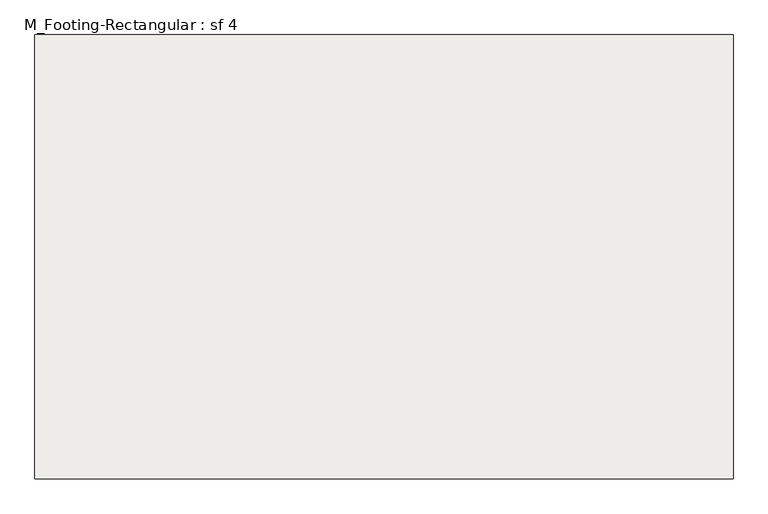
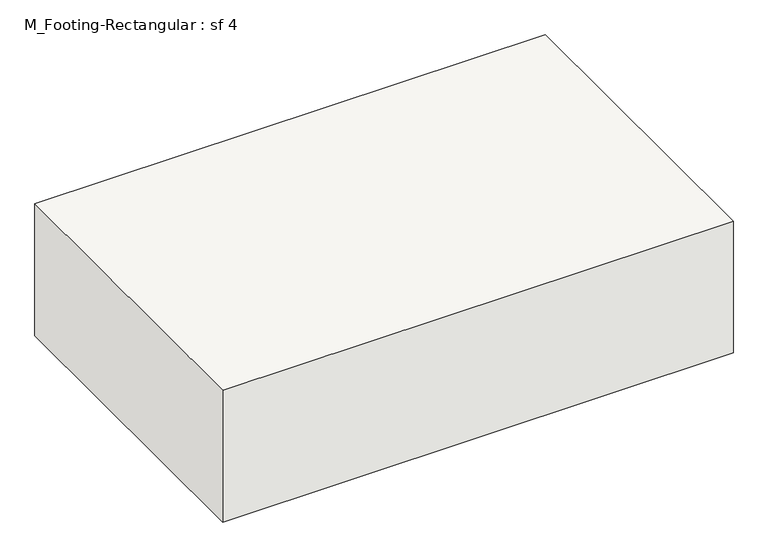
"""IFC4 building model written with IfcOpenShell, lengths in millimetres: slab geometry, M_Footing-Rectangular : sf 4."""

from ifc_helpers import new_model, si_unit, frame, origin, place, context, project, spatial, polyline, outline, extrude, source, transform, mapped, element, save


def m_footing_rectangular_sf_4_edbcb53e(model_context):
    return source(origin(), model_context, "Body", "SweptSolid", [
        extrude(outline(polyline([(838.2, 533.4), (838.2, -533.4), (-838.2, -533.4), (-838.2, 533.4), (838.2, 533.4)])), frame((0.0, 0.0, -457.2), z_axis=(0.0, 0.0, 1.0), x_axis=(1.0, 0.0, 0.0)), (0.0, 0.0, 1.0), 457.2),
    ])


if __name__ == "__main__":
    model = new_model("IFC4")
    model_context = context("Model", 3, world=origin())
    ifc_project = project(units=[si_unit("LENGTHUNIT", "METRE", prefix="MILLI")], contexts=[model_context])
    site = spatial("IfcSite", under=ifc_project)
    building = spatial("IfcBuilding", under=site)
    placement = place(None, origin())
    m_footing_rectangular_sf_4_shape = m_footing_rectangular_sf_4_edbcb53e(model_context)
    element("IfcSlab", 1, ObjectType="M_Footing-Rectangular : sf 4", at=placement, inside=building, context=model_context, shape_type="MappedRepresentation", body=[
        mapped(m_footing_rectangular_sf_4_shape, transform((0.0, 0.0, 0.0), x_axis=(1.0, 0.0, 0.0), y_axis=(0.0, 1.0, 0.0), z_axis=(0.0, 0.0, 1.0))),
    ])
    save(model, "model.ifc")

# Revit data of these elements
# Type "M_Footing-Rectangular : sf 4"
#   Width = 1676.4 mm
#   Length = 1066.8 mm
#   Foundation Thickness = 457.2 mm
#   Structural Material [instance default] = Concrete, Cast-in-Place gray
#   Assembly Code = ""
# Element 1 (IfcSlab, "M_Footing-Rectangular : sf 4")
#   Materials on its faces: "Concrete, Cast-in-Place gray"
# Materials
#   "Concrete, Cast-in-Place gray": class "Concrete", colour RGB 192 192 192, transparency 0, Description = "Cast-in-place concrete", Cost = 0
